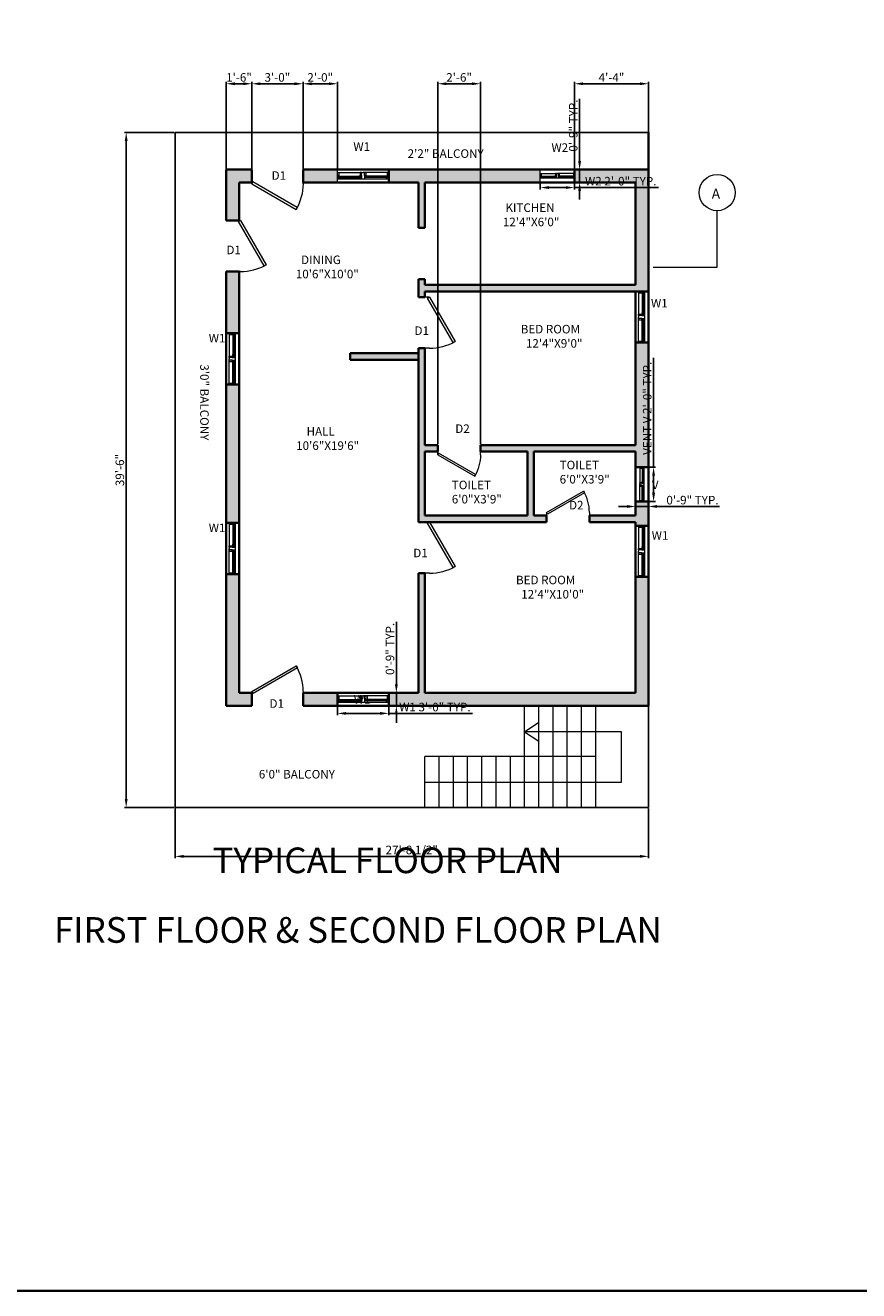
# Model space of a CAD drawing. Units: millimetres. Extents: x 50579 to 52843, y 62224 to 63803.
# Tile 3 of 5: x 51453 to 52038, y 62224 to 63113. Entities that reach past the tile are written whole.
import ezdxf

# ---------------------------------------------------------------- set-up
doc = ezdxf.new("R2010")
doc.units = ezdxf.units.MM
for name, color, linetype, lineweight in [('A-ANNO-DIMS', 2, 'Continuous', 18), ('A-ANNO-IDEN', 6, 'Continuous', 18), ('A-ANNO-SYMB', 6, 'Continuous', 18), ('A-ANNO-TITL', 4, 'Continuous', 25), ('A-ANNO-TTLB', 7, 'Continuous', 35), ('A-AREA-IDEN', 6, 'Continuous', 18), ('A-FLOR-BALC', 7, 'Continuous', 25), ('A-FLOR-STRS', 7, 'Continuous', 18), ('A-GLAZ', 4, 'Continuous', 18), ('A-WALL', 7, 'Continuous', 35), ('A-WALL-PATT', 251, 'Continuous', 13), ('DOOR', 20, 'Continuous', 18)]:
    doc.layers.add(name, color=color, linetype=linetype, lineweight=lineweight)
doc.styles.get("Standard").update_dxf_attribs({"font": 'arial.ttf'})
doc.dimstyles.new('ISO-25', dxfattribs={"dimtxt": 6, "dimasz": 6, "dimexe": 1.25, "dimexo": 0.625, "dimtad": 1, "dimdec": 0, "dimlunit": 3, "dimtxsty": 'Standard', "dimcen": 2.5, "dimadec": 0, "dimazin": 0, "dimtfac": 1, "dimtdec": 0, "dimtmove": 0, "dimatfit": 3, "dimfxl": 1, "dimarcsym": 0})

# ---------------------------------------------------------------- blocks, each defined once
blk = doc.blocks.new('W1')
for p, q in [((50927.56, 62719.85), (50945.56, 62719.85)), ((50927.56, 62717.25), (50944.56, 62717.25)), ((50927.56, 62716.35), (50944.56, 62716.35)), ((50927.56, 62715.35), (50963.56, 62715.35)), ((50929.58, 62717.08), (50942.53, 62717.08)), ((50929.58, 62716.8), (50942.53, 62716.8)), ((50929.58, 62716.54), (50942.53, 62716.54)), ((50944.56, 62717.61), (50944.56, 62715.35)), ((50963.56, 62719.85), (50945.56, 62719.85)), ((50946.56, 62717.61), (50946.56, 62715.35)), ((50963.56, 62717.25), (50946.56, 62717.25)), ((50963.56, 62716.35), (50946.56, 62716.35)), ((50961.53, 62717.08), (50948.58, 62717.08)), ((50961.53, 62716.8), (50948.58, 62716.8)), ((50961.53, 62716.54), (50948.58, 62716.54))]:
    blk.add_line(p, q)
for points in [[(50927.56, 62712.85), (50927.56, 62721.85), (50963.56, 62721.85), (50963.56, 62712.85)], [(50927.56, 62719.85), (50928.5, 62719.85), (50928.5, 62717.61), (50927.56, 62717.61)], [(50928.59, 62717.25), (50929.58, 62717.25), (50929.58, 62716.35), (50928.59, 62716.35)], [(50943.52, 62717.25), (50942.53, 62717.25), (50942.53, 62716.35), (50943.52, 62716.35)], [(50944.56, 62719.85), (50943.61, 62719.85), (50943.61, 62717.61), (50944.56, 62717.61)], [(50946.56, 62719.85), (50947.5, 62719.85), (50947.5, 62717.61), (50946.56, 62717.61)], [(50947.59, 62717.25), (50948.58, 62717.25), (50948.58, 62716.35), (50947.59, 62716.35)], [(50962.52, 62717.25), (50961.53, 62717.25), (50961.53, 62716.35), (50962.52, 62716.35)], [(50963.56, 62719.85), (50962.61, 62719.85), (50962.61, 62717.61), (50963.56, 62717.61)]]:
    blk.add_lwpolyline(points, close=True)
blk = doc.blocks.new('*U3')
for p, q in [((0, 0), (0, -6)), ((40, 0), (40, -6))]:
    blk.add_line(p, q)
blk.add_lwpolyline([(0, 0), (34.64, 20), (35.52, 18.48), (0.87, -1.52)], close=True)
blk.add_arc((0, 0), 40, 0, 30)
blk = doc.blocks.new('WIN-W2-PLAN')
for p, q in [((0, 6.16), (12, 6.16)), ((0, 4.43), (11.33, 4.43)), ((0, 3.83), (11.33, 3.83)), ((0, 3.16), (24, 3.16)), ((1.35, 4.32), (9.98, 4.32)), ((1.35, 4.13), (9.98, 4.13)), ((1.35, 3.95), (9.98, 3.95)), ((11.33, 4.67), (11.33, 3.16)), ((24, 6.16), (12, 6.16)), ((12.67, 4.67), (12.67, 3.16)), ((24, 4.43), (12.67, 4.43)), ((24, 3.83), (12.67, 3.83)), ((22.65, 4.32), (14.02, 4.32)), ((22.65, 4.13), (14.02, 4.13)), ((22.65, 3.95), (14.02, 3.95))]:
    blk.add_line(p, q)
for points in [[(0, 0), (0, 9), (24, 9), (24, 0)], [(0, 6.16), (0.63, 6.16), (0.63, 4.67), (0, 4.67)], [(0.69, 4.43), (1.35, 4.43), (1.35, 3.83), (0.69, 3.83)], [(10.64, 4.43), (9.98, 4.43), (9.98, 3.83), (10.64, 3.83)], [(11.33, 6.16), (10.7, 6.16), (10.7, 4.67), (11.33, 4.67)], [(12.67, 6.16), (13.29, 6.16), (13.29, 4.67), (12.67, 4.67)], [(13.36, 4.43), (14.02, 4.43), (14.02, 3.83), (13.36, 3.83)], [(23.31, 4.43), (22.65, 4.43), (22.65, 3.83), (23.31, 3.83)], [(24, 6.16), (23.37, 6.16), (23.37, 4.67), (24, 4.67)]]:
    blk.add_lwpolyline(points, close=True)
blk = doc.blocks.new('VENT-V-PLAN')
for p, q in [((2.84, 24), (2.84, 12)), ((4.57, 24), (4.57, 12.67)), ((4.68, 22.65), (4.68, 14.02)), ((4.87, 22.65), (4.87, 14.02)), ((5.05, 22.65), (5.05, 14.02)), ((5.17, 24), (5.17, 12.67)), ((5.84, 24), (5.84, 0)), ((2.84, 0), (2.84, 12)), ((4.33, 12.67), (5.84, 12.67)), ((4.33, 11.33), (5.84, 11.33)), ((4.57, 0), (4.57, 11.33)), ((4.68, 1.35), (4.68, 9.98)), ((4.87, 1.35), (4.87, 9.98)), ((5.05, 1.35), (5.05, 9.98)), ((5.17, 0), (5.17, 11.33))]:
    blk.add_line(p, q)
for points in [[(9, 24), (0, 24), (0, 0), (9, 0)], [(2.84, 24), (2.84, 23.37), (4.33, 23.37), (4.33, 24)], [(4.57, 23.31), (4.57, 22.65), (5.17, 22.65), (5.17, 23.31)], [(2.84, 12.67), (2.84, 13.3), (4.33, 13.3), (4.33, 12.67)], [(2.84, 11.33), (2.84, 10.71), (4.33, 10.71), (4.33, 11.33)], [(4.57, 13.36), (4.57, 14.02), (5.17, 14.02), (5.17, 13.36)], [(4.57, 10.64), (4.57, 9.98), (5.17, 9.98), (5.17, 10.64)], [(2.84, 0), (2.84, 0.63), (4.33, 0.63), (4.33, 0)], [(4.57, 0.69), (4.57, 1.35), (5.17, 1.35), (5.17, 0.69)]]:
    blk.add_lwpolyline(points, close=True)
blk = doc.blocks.new('STAIR-RETURN-PLAN')
for p, q in [((70, 0), (70, 71.5)), ((80, 0), (80, 71.5)), ((90, 0), (90, 71.5)), ((100, 0), (100, 71.5)), ((110, 0), (110, 71.5)), ((120, 0), (120, 71.5)), ((70, 53.25), (80, 59.99)), ((138.14, 53.25), (70, 53.25)), ((70, 53.25), (80, 46.5)), ((138.14, 17.87), (138.14, 53.25)), ((0, 0), (0, 35.75)), ((120, 35.75), (0, 35.75)), ((10, 0), (10, 35.75)), ((20, 0), (20, 35.75)), ((30, 0), (30, 35.75)), ((40, 0), (40, 35.75)), ((50, 0), (50, 35.75)), ((60, 0), (60, 35.75)), ((0, 17.87), (138.14, 17.87))]:
    blk.add_line(p, q)
blk = doc.blocks.new('*D27')
at = {"layer": 'A-ANNO-DIMS', "color": 0, "lineweight": -2, "transparency": 16777216}
for p, q in [((51671.96, 62634.23), (51671.96, 62628.2)), ((51707.96, 62634.23), (51707.96, 62628.2)), ((51677.96, 62629.45), (51701.96, 62629.45)), ((51707.96, 62629.45), (51766.93, 62629.45))]:
    blk.add_line(p, q, dxfattribs=at)
at = {"layer": 'A-ANNO-DIMS', "color": 0, "transparency": 16777216}
for points in [[(51677.96, 62630.45), (51677.96, 62628.45), (51671.96, 62629.45)], [(51701.96, 62630.45), (51701.96, 62628.45), (51707.96, 62629.45)]]:
    blk.add_solid(points, dxfattribs=at)
at = {"layer": 'Defpoints', "color": 0, "transparency": 16777216}
for p in [(51671.96, 62634.85), (51707.96, 62634.85), (51707.96, 62629.45)]:
    blk.add_point(p, dxfattribs=at)
at = {"layer": 'A-ANNO-DIMS', "color": 0, "transparency": 16777216, "insert": (51740.44, 62633.14), "char_height": 6, "attachment_point": 5}
blk.add_mtext('W1 3\'-0" TYP.', dxfattribs=at)
blk = doc.blocks.new('*D28')
at = {"layer": 'A-ANNO-DIMS', "color": 0, "lineweight": -2, "transparency": 16777216}
for p, q in [((51713.36, 62649.85), (51713.36, 62693.67)), ((51708.58, 62643.85), (51714.61, 62643.85)), ((51713.36, 62634.85), (51713.36, 62643.85)), ((51708.58, 62634.85), (51714.61, 62634.85)), ((51713.36, 62628.85), (51713.36, 62622.85))]:
    blk.add_line(p, q, dxfattribs=at)
at = {"layer": 'A-ANNO-DIMS', "color": 0, "transparency": 16777216}
for points in [[(51712.36, 62649.85), (51714.36, 62649.85), (51713.36, 62643.85)], [(51712.36, 62628.85), (51714.36, 62628.85), (51713.36, 62634.85)]]:
    blk.add_solid(points, dxfattribs=at)
at = {"layer": 'Defpoints', "color": 0, "transparency": 16777216}
for p in [(51707.96, 62643.85), (51713.36, 62643.85), (51707.96, 62634.85)]:
    blk.add_point(p, dxfattribs=at)
at = {"layer": 'A-ANNO-DIMS', "color": 0, "transparency": 16777216, "insert": (51709.67, 62674.76), "char_height": 6, "attachment_point": 5, "rotation": 90}
blk.add_mtext('0\'-9" TYP.', dxfattribs=at)
blk = doc.blocks.new('*D29')
at = {"layer": 'A-ANNO-DIMS', "color": 0, "lineweight": -2, "transparency": 16777216}
for p, q in [((51814.46, 63001.73), (51814.46, 62997.5)), ((51820.46, 62998.75), (51832.46, 62998.75)), ((51838.46, 63001.73), (51838.46, 62997.5)), ((51838.46, 62998.75), (51897.43, 62998.75))]:
    blk.add_line(p, q, dxfattribs=at)
at = {"layer": 'A-ANNO-DIMS', "color": 0, "transparency": 16777216}
for points in [[(51820.46, 62999.75), (51820.46, 62997.75), (51814.46, 62998.75)], [(51832.46, 62999.75), (51832.46, 62997.75), (51838.46, 62998.75)]]:
    blk.add_solid(points, dxfattribs=at)
at = {"layer": 'Defpoints', "color": 0, "transparency": 16777216}
for p in [(51814.46, 63002.35), (51838.46, 63002.35), (51838.46, 62998.75)]:
    blk.add_point(p, dxfattribs=at)
at = {"layer": 'A-ANNO-DIMS', "color": 0, "transparency": 16777216, "insert": (51870.94, 63002.44), "char_height": 6, "attachment_point": 5}
blk.add_mtext('W2 2\'-0" TYP.', dxfattribs=at)
blk = doc.blocks.new('*D30')
at = {"layer": 'A-ANNO-DIMS', "color": 0, "lineweight": -2, "transparency": 16777216}
for p, q in [((51842.06, 63017.35), (51842.06, 63061.17)), ((51839.08, 63011.35), (51843.31, 63011.35)), ((51842.06, 63002.35), (51842.06, 63011.35)), ((51839.08, 63002.35), (51843.31, 63002.35)), ((51842.06, 62996.35), (51842.06, 62990.35))]:
    blk.add_line(p, q, dxfattribs=at)
at = {"layer": 'A-ANNO-DIMS', "color": 0, "transparency": 16777216}
for points in [[(51841.06, 63017.35), (51843.06, 63017.35), (51842.06, 63011.35)], [(51841.06, 62996.35), (51843.06, 62996.35), (51842.06, 63002.35)]]:
    blk.add_solid(points, dxfattribs=at)
at = {"layer": 'Defpoints', "color": 0, "transparency": 16777216}
for p in [(51838.46, 63011.35), (51842.06, 63011.35), (51838.46, 63002.35)]:
    blk.add_point(p, dxfattribs=at)
at = {"layer": 'A-ANNO-DIMS', "color": 0, "transparency": 16777216, "insert": (51838.37, 63042.26), "char_height": 6, "attachment_point": 5, "rotation": 90}
blk.add_mtext('0\'-9" TYP.', dxfattribs=at)
blk = doc.blocks.new('*D31')
at = {"layer": 'A-ANNO-DIMS', "color": 0, "lineweight": -2, "transparency": 16777216}
for p, q in [((51894.02, 62802.37), (51894.02, 62879.11)), ((51891.04, 62802.37), (51895.27, 62802.37)), ((51894.02, 62784.37), (51894.02, 62796.37)), ((51891.04, 62778.37), (51895.27, 62778.37))]:
    blk.add_line(p, q, dxfattribs=at)
at = {"layer": 'A-ANNO-DIMS', "color": 0, "transparency": 16777216}
for points in [[(51893.02, 62796.37), (51895.02, 62796.37), (51894.02, 62802.37)], [(51893.02, 62784.37), (51895.02, 62784.37), (51894.02, 62778.37)]]:
    blk.add_solid(points, dxfattribs=at)
at = {"layer": 'Defpoints', "color": 0, "transparency": 16777216}
for p in [(51890.42, 62802.37), (51894.02, 62802.37), (51890.42, 62778.37)]:
    blk.add_point(p, dxfattribs=at)
at = {"layer": 'A-ANNO-DIMS', "color": 0, "transparency": 16777216, "insert": (51890.33, 62843.74), "char_height": 6, "attachment_point": 5, "rotation": 90}
blk.add_mtext('VENT V 2\'-0" TYP.', dxfattribs=at)
blk = doc.blocks.new('*D32')
at = {"layer": 'A-ANNO-DIMS', "color": 0, "lineweight": -2, "transparency": 16777216}
for p, q in [((51881.42, 62777.75), (51881.42, 62773.52)), ((51890.42, 62777.75), (51890.42, 62773.52)), ((51875.42, 62774.77), (51869.42, 62774.77)), ((51881.42, 62774.77), (51890.42, 62774.77)), ((51896.42, 62774.77), (51940.24, 62774.77))]:
    blk.add_line(p, q, dxfattribs=at)
at = {"layer": 'A-ANNO-DIMS', "color": 0, "transparency": 16777216}
for points in [[(51875.42, 62775.77), (51875.42, 62773.77), (51881.42, 62774.77)], [(51896.42, 62775.77), (51896.42, 62773.77), (51890.42, 62774.77)]]:
    blk.add_solid(points, dxfattribs=at)
at = {"layer": 'Defpoints', "color": 0, "transparency": 16777216}
for p in [(51881.42, 62778.37), (51890.42, 62778.37), (51890.42, 62774.77)]:
    blk.add_point(p, dxfattribs=at)
at = {"layer": 'A-ANNO-DIMS', "color": 0, "transparency": 16777216, "insert": (51921.33, 62778.46), "char_height": 6, "attachment_point": 5}
blk.add_mtext('0\'-9" TYP.', dxfattribs=at)
blk = doc.blocks.new('*D41')
at = {"layer": 'A-ANNO-DIMS', "color": 0, "lineweight": -2, "transparency": 16777216}
for p, q in [((51557.92, 62562.73), (51557.92, 62527.8)), ((51890.42, 62562.73), (51890.42, 62527.8)), ((51563.92, 62529.05), (51884.42, 62529.05))]:
    blk.add_line(p, q, dxfattribs=at)
at = {"layer": 'A-ANNO-DIMS', "color": 0, "transparency": 16777216}
for points in [[(51563.92, 62530.05), (51563.92, 62528.05), (51557.92, 62529.05)], [(51884.42, 62530.05), (51884.42, 62528.05), (51890.42, 62529.05)]]:
    blk.add_solid(points, dxfattribs=at)
at = {"layer": 'Defpoints', "color": 0, "transparency": 16777216}
for p in [(51557.92, 62563.35), (51890.42, 62563.35), (51890.42, 62529.05)]:
    blk.add_point(p, dxfattribs=at)
at = {"layer": 'A-ANNO-DIMS', "color": 0, "transparency": 16777216, "insert": (51724.17, 62532.78), "char_height": 6, "attachment_point": 5}
blk.add_mtext('27\'-8 1/2"', dxfattribs=at)
blk = doc.blocks.new('*D42')
at = {"layer": 'A-ANNO-DIMS', "color": 0, "lineweight": -2, "transparency": 16777216}
for p, q in [((51557.29, 63037.35), (51522.37, 63037.35)), ((51523.62, 62569.35), (51523.62, 63031.35)), ((51557.29, 62563.35), (51522.37, 62563.35))]:
    blk.add_line(p, q, dxfattribs=at)
at = {"layer": 'A-ANNO-DIMS', "color": 0, "transparency": 16777216}
for points in [[(51522.62, 63031.35), (51524.62, 63031.35), (51523.62, 63037.35)], [(51522.62, 62569.35), (51524.62, 62569.35), (51523.62, 62563.35)]]:
    blk.add_solid(points, dxfattribs=at)
at = {"layer": 'Defpoints', "color": 0, "transparency": 16777216}
for p in [(51523.62, 63037.35), (51557.92, 63037.35), (51557.92, 62563.35)]:
    blk.add_point(p, dxfattribs=at)
at = {"layer": 'A-ANNO-DIMS', "color": 0, "transparency": 16777216, "insert": (51519.93, 62800.35), "char_height": 6, "attachment_point": 5, "rotation": 90}
blk.add_mtext('39\'-6"', dxfattribs=at)
blk = doc.blocks.new('*D68')
at = {"layer": 'A-ANNO-DIMS', "color": 0, "lineweight": -2, "transparency": 16777216}
for p, q in [((51611.8, 63011.98), (51611.8, 63072.9)), ((51617.8, 63071.65), (51641.8, 63071.65)), ((51647.8, 63011.98), (51647.8, 63072.9))]:
    blk.add_line(p, q, dxfattribs=at)
at = {"layer": 'A-ANNO-DIMS', "color": 0, "transparency": 16777216}
for points in [[(51617.8, 63072.65), (51617.8, 63070.65), (51611.8, 63071.65)], [(51641.8, 63072.65), (51641.8, 63070.65), (51647.8, 63071.65)]]:
    blk.add_solid(points, dxfattribs=at)
at = {"layer": 'Defpoints', "color": 0, "transparency": 16777216}
for p in [(51647.8, 63071.65), (51611.8, 63011.35), (51647.8, 63011.35)]:
    blk.add_point(p, dxfattribs=at)
at = {"layer": 'A-ANNO-DIMS', "color": 0, "transparency": 16777216, "insert": (51629.8, 63075.34), "char_height": 6, "attachment_point": 5}
blk.add_mtext('3\'-0"', dxfattribs=at)
blk = doc.blocks.new('*D69')
at = {"layer": 'A-ANNO-DIMS', "color": 0, "lineweight": -2, "transparency": 16777216}
for p, q in [((51742.42, 62818.48), (51742.42, 63072.9)), ((51748.42, 63071.65), (51766.42, 63071.65)), ((51772.42, 62818.48), (51772.42, 63072.9))]:
    blk.add_line(p, q, dxfattribs=at)
at = {"layer": 'A-ANNO-DIMS', "color": 0, "transparency": 16777216}
for points in [[(51748.42, 63072.65), (51748.42, 63070.65), (51742.42, 63071.65)], [(51766.42, 63072.65), (51766.42, 63070.65), (51772.42, 63071.65)]]:
    blk.add_solid(points, dxfattribs=at)
at = {"layer": 'Defpoints', "color": 0, "transparency": 16777216}
for p in [(51772.42, 63071.65), (51742.42, 62817.85), (51772.42, 62817.85)]:
    blk.add_point(p, dxfattribs=at)
at = {"layer": 'A-ANNO-DIMS', "color": 0, "transparency": 16777216, "insert": (51757.42, 63075.34), "char_height": 6, "attachment_point": 5}
blk.add_mtext('2\'-6"', dxfattribs=at)
blk = doc.blocks.new('*D70')
at = {"layer": 'A-ANNO-DIMS', "color": 0, "lineweight": -2, "transparency": 16777216}
for p, q in [((51593.92, 63011.98), (51593.92, 63072.9)), ((51599.92, 63071.65), (51605.8, 63071.65)), ((51611.8, 63011.98), (51611.8, 63072.9))]:
    blk.add_line(p, q, dxfattribs=at)
at = {"layer": 'A-ANNO-DIMS', "color": 0, "transparency": 16777216}
for points in [[(51599.92, 63072.65), (51599.92, 63070.65), (51593.92, 63071.65)], [(51605.8, 63072.65), (51605.8, 63070.65), (51611.8, 63071.65)]]:
    blk.add_solid(points, dxfattribs=at)
at = {"layer": 'Defpoints', "color": 0, "transparency": 16777216}
for p in [(51611.8, 63071.65), (51593.92, 63011.35), (51611.8, 63011.35)]:
    blk.add_point(p, dxfattribs=at)
at = {"layer": 'A-ANNO-DIMS', "color": 0, "transparency": 16777216, "insert": (51602.86, 63075.34), "char_height": 6, "attachment_point": 5}
blk.add_mtext('1\'-6"', dxfattribs=at)
blk = doc.blocks.new('*D71')
at = {"layer": 'A-ANNO-DIMS', "color": 0, "lineweight": -2, "transparency": 16777216}
for p, q in [((51647.8, 63011.98), (51647.8, 63072.9)), ((51653.8, 63071.65), (51665.96, 63071.65)), ((51671.96, 63011.98), (51671.96, 63072.9))]:
    blk.add_line(p, q, dxfattribs=at)
at = {"layer": 'A-ANNO-DIMS', "color": 0, "transparency": 16777216}
for points in [[(51653.8, 63072.65), (51653.8, 63070.65), (51647.8, 63071.65)], [(51665.96, 63072.65), (51665.96, 63070.65), (51671.96, 63071.65)]]:
    blk.add_solid(points, dxfattribs=at)
at = {"layer": 'Defpoints', "color": 0, "transparency": 16777216}
for p in [(51671.96, 63071.65), (51647.8, 63011.35), (51671.96, 63011.35)]:
    blk.add_point(p, dxfattribs=at)
at = {"layer": 'A-ANNO-DIMS', "color": 0, "transparency": 16777216, "insert": (51659.88, 63075.34), "char_height": 6, "attachment_point": 5}
blk.add_mtext('2\'-0"', dxfattribs=at)
blk = doc.blocks.new('*D72')
at = {"layer": 'A-ANNO-DIMS', "color": 0, "lineweight": -2, "transparency": 16777216}
for p, q in [((51838.455361, 63011.976927), (51838.455361, 63072.901927)), ((51844.455361, 63071.651927), (51884.419171, 63071.651927)), ((51890.419171, 63011.976927), (51890.419171, 63072.901927))]:
    blk.add_line(p, q, dxfattribs=at)
at = {"layer": 'A-ANNO-DIMS', "color": 0, "transparency": 16777216}
for points in [[(51844.455361, 63072.651927), (51844.455361, 63070.651927), (51838.455361, 63071.651927)], [(51884.419171, 63072.651927), (51884.419171, 63070.651927), (51890.419171, 63071.651927)]]:
    blk.add_solid(points, dxfattribs=at)
at = {"layer": 'Defpoints', "color": 0, "transparency": 16777216}
for p in [(51890.419171, 63071.651927), (51838.455361, 63011.351927), (51890.419171, 63011.351927)]:
    blk.add_point(p, dxfattribs=at)
at = {"layer": 'A-ANNO-DIMS', "color": 0, "transparency": 16777216, "insert": (51864.437266, 63075.276927), "char_height": 6, "attachment_point": 5}
blk.add_mtext('4\'-4"', dxfattribs=at)

msp = doc.modelspace()

# ---------------------------------------------------------------- hatches: boundary and pattern name
at = {"layer": 'A-WALL-PATT'}
h = msp.add_hatch(color=256, dxfattribs=at)
h.dxf.hatch_style = 1
h.paths.add_polyline_path([(51611.8, 63006.85), (51611.8, 63011.35), (51593.92, 63011.35), (51593.92, 62975.7), (51602.92, 62975.7), (51602.92, 63002.35), (51611.8, 63002.35)])
h = msp.add_hatch(color=256, dxfattribs=at)
h.dxf.hatch_style = 1
h.paths.add_polyline_path([(51671.96, 63011.35), (51647.8, 63011.35), (51647.8, 63002.35), (51671.96, 63002.35)])
h = msp.add_hatch(color=256, dxfattribs=at)
h.dxf.hatch_style = 1
h.paths.add_polyline_path([(51814.46, 63011.35), (51707.96, 63011.35), (51707.96, 63002.35), (51728.92, 63002.35), (51728.92, 62970.35), (51733.42, 62970.35), (51733.42, 63002.35), (51814.46, 63002.35)])
h = msp.add_hatch(color=256, dxfattribs=at)
h.dxf.hatch_style = 1
h.paths.add_polyline_path([(51890.42, 63011.35), (51838.46, 63011.35), (51838.46, 63002.35), (51881.42, 63002.35), (51881.42, 62930.35), (51733.42, 62930.35), (51733.42, 62934.35), (51728.92, 62934.35), (51728.92, 62921.85), (51733.42, 62921.85), (51733.42, 62925.85), (51890.42, 62925.85)])
h = msp.add_hatch(color=256, dxfattribs=at)
h.dxf.hatch_style = 1
h.paths.add_polyline_path([(51602.92, 62939.7), (51598.42, 62939.7), (51593.92, 62939.7), (51593.92, 62896.5), (51602.92, 62896.5)])
h = msp.add_hatch(color=256, dxfattribs=at)
h.dxf.hatch_style = 1
h.paths.add_polyline_path([(51728.92, 62882.35), (51680.92, 62882.35), (51680.92, 62877.85), (51728.92, 62877.85)])
h = msp.add_hatch(color=256, dxfattribs=at)
h.dxf.hatch_style = 1
h.paths.add_polyline_path([(51733.42, 62885.85), (51731.17, 62885.85), (51728.92, 62885.85), (51728.92, 62763.85), (51818.92, 62763.85), (51818.92, 62768.35), (51809.92, 62768.35), (51809.92, 62813.35), (51881.42, 62813.35), (51881.42, 62802.37), (51890.42, 62802.37), (51890.42, 62889.85), (51881.42, 62889.85), (51881.42, 62817.85), (51772.42, 62817.85), (51772.42, 62813.35), (51805.42, 62813.35), (51805.42, 62768.35), (51733.42, 62768.35), (51733.42, 62813.35), (51742.42, 62813.35), (51742.42, 62815.6), (51742.42, 62817.85), (51733.42, 62817.85)])
h = msp.add_hatch(color=256, dxfattribs=at)
h.dxf.hatch_style = 1
h.paths.add_polyline_path([(51602.92, 62860.5), (51593.92, 62860.5), (51593.92, 62763.3), (51602.92, 62763.3)])
h = msp.add_hatch(color=256, dxfattribs=at)
h.dxf.hatch_style = 1
h.paths.add_polyline_path([(51890.42, 62778.37), (51881.42, 62778.37), (51881.42, 62768.35), (51848.92, 62768.35), (51848.92, 62763.85), (51881.42, 62763.85), (51881.42, 62761.3), (51890.42, 62761.3)])
h = msp.add_hatch(color=256, dxfattribs=at)
h.dxf.hatch_style = 1
h.paths.add_polyline_path([(51611.92, 62643.85), (51602.92, 62643.85), (51602.92, 62727.3), (51593.92, 62727.3), (51593.92, 62643.85), (51593.92, 62634.85), (51611.92, 62634.85)])
h = msp.add_hatch(color=256, dxfattribs=at)
h.dxf.hatch_style = 1
h.paths.add_polyline_path([(51890.42, 62725.3), (51881.42, 62725.3), (51881.42, 62643.85), (51733.42, 62643.85), (51733.42, 62727.85), (51728.92, 62727.85), (51728.92, 62643.85), (51707.96, 62643.85), (51707.96, 62634.85), (51890.42, 62634.85)])
h = msp.add_hatch(color=256, dxfattribs=at)
h.dxf.hatch_style = 1
h.paths.add_polyline_path([(51671.96, 62643.85), (51647.92, 62643.85), (51647.92, 62634.85), (51671.96, 62634.85)])

# ---------------------------------------------------------------- linework, layer by layer
at = {"layer": 'A-ANNO-SYMB'}
for p, q in [((51938.69, 62942.81), (51938.69, 62982.48)), ((51893.74, 62942.81), (51938.69, 62942.81))]:
    msp.add_line(p, q, dxfattribs=at)
msp.add_circle((51938.69, 62995.17), 12.7, dxfattribs=at)
at = {"layer": 'A-ANNO-TTLB'}
msp.add_lwpolyline([(50579.46, 63802.65), (52843.1, 63802.65), (52843.1, 62224.04), (50579.46, 62224.04)], close=True, dxfattribs=at)
at = {"layer": 'A-FLOR-BALC'}
for p, q in [((51557.92, 63037.35), (51890.42, 63037.35)), ((51557.92, 62563.35), (51557.92, 63037.35)), ((51890.42, 62634.85), (51890.42, 62563.35)), ((51890.42, 62563.35), (51557.92, 62563.35))]:
    msp.add_line(p, q, dxfattribs=at)
at = {"layer": 'A-WALL'}
for p, q in [((51890.42, 62634.85), (51890.42, 63037.35)), ((51593.92, 63011.35), (51611.8, 63011.35)), ((51593.92, 62975.7), (51593.92, 63011.35)), ((51611.8, 63002.35), (51611.8, 63011.35)), ((51647.8, 63011.35), (51890.42, 63011.35)), ((51647.8, 63002.35), (51647.8, 63011.35)), ((51707.96, 63011.35), (51707.96, 63002.35)), ((51838.46, 63011.35), (51838.46, 63002.35)), ((51602.92, 63002.35), (51611.8, 63002.35)), ((51602.92, 62975.7), (51602.92, 63002.35)), ((51647.8, 63002.35), (51728.92, 63002.35)), ((51728.92, 62970.35), (51728.92, 63002.35)), ((51733.42, 63002.35), (51881.42, 63002.35)), ((51733.42, 62970.35), (51733.42, 63002.35)), ((51881.42, 62930.35), (51881.42, 63002.35)), ((51593.92, 62975.7), (51602.92, 62975.7)), ((51728.92, 62970.35), (51733.42, 62970.35)), ((51593.92, 62643.85), (51593.92, 62939.7)), ((51593.92, 62939.7), (51602.92, 62939.7)), ((51602.92, 62877.85), (51602.92, 62939.7)), ((51728.92, 62934.35), (51733.42, 62934.35)), ((51728.92, 62921.85), (51728.92, 62934.35)), ((51733.42, 62930.35), (51733.42, 62934.35)), ((51733.42, 62930.35), (51881.42, 62930.35)), ((51733.42, 62925.85), (51890.42, 62925.85)), ((51733.42, 62921.85), (51733.42, 62925.85)), ((51881.42, 62817.85), (51881.42, 62925.85)), ((51728.92, 62921.85), (51733.42, 62921.85)), ((51593.92, 62896.5), (51602.92, 62896.5)), ((51680.92, 62882.35), (51728.92, 62882.35)), ((51680.92, 62877.85), (51680.92, 62882.35)), ((51728.92, 62885.85), (51733.42, 62885.85)), ((51728.92, 62763.85), (51728.92, 62885.85)), ((51733.42, 62817.85), (51733.42, 62885.85)), ((51881.42, 62889.85), (51890.42, 62889.85)), ((51602.92, 62643.85), (51602.92, 62877.85)), ((51680.92, 62877.85), (51728.92, 62877.85)), ((51593.92, 62860.5), (51602.92, 62860.5)), ((51733.42, 62817.85), (51742.42, 62817.85)), ((51733.42, 62813.35), (51742.42, 62813.35)), ((51733.42, 62768.35), (51733.42, 62813.35)), ((51742.42, 62813.35), (51742.42, 62817.85)), ((51772.42, 62817.85), (51881.42, 62817.85)), ((51772.42, 62813.35), (51772.42, 62817.85)), ((51772.42, 62813.35), (51805.42, 62813.35)), ((51805.42, 62768.35), (51805.42, 62813.35)), ((51809.92, 62813.35), (51881.42, 62813.35)), ((51809.92, 62768.35), (51809.92, 62813.35)), ((51881.42, 62768.35), (51881.42, 62813.35)), ((51881.42, 62802.37), (51890.42, 62802.37)), ((51881.42, 62778.37), (51890.42, 62778.37)), ((51733.42, 62768.35), (51805.42, 62768.35)), ((51809.92, 62768.35), (51818.92, 62768.35)), ((51818.92, 62768.35), (51818.92, 62763.85)), ((51848.92, 62768.35), (51881.42, 62768.35)), ((51848.92, 62768.35), (51848.92, 62763.85)), ((51593.92, 62763.3), (51602.92, 62763.3)), ((51728.92, 62763.85), (51818.92, 62763.85)), ((51848.92, 62763.85), (51881.42, 62763.85)), ((51881.42, 62643.85), (51881.42, 62763.85)), ((51881.42, 62761.3), (51890.42, 62761.3)), ((51593.92, 62727.3), (51602.92, 62727.3)), ((51728.92, 62727.85), (51733.42, 62727.85)), ((51728.92, 62643.85), (51728.92, 62727.85)), ((51733.42, 62643.85), (51733.42, 62727.85)), ((51881.42, 62725.3), (51890.42, 62725.3)), ((51593.92, 62634.85), (51593.92, 62643.85)), ((51602.92, 62643.85), (51611.92, 62643.85)), ((51611.92, 62643.85), (51611.92, 62634.85)), ((51647.92, 62643.85), (51647.92, 62634.85)), ((51647.92, 62643.85), (51728.92, 62643.85)), ((51671.96, 62643.85), (51671.96, 62634.85)), ((51707.96, 62643.85), (51707.96, 62634.85)), ((51733.42, 62643.85), (51881.42, 62643.85)), ((51593.92, 62634.85), (51611.92, 62634.85)), ((51647.92, 62634.85), (51890.42, 62634.85))]:
    msp.add_line(p, q, dxfattribs=at)

# ---------------------------------------------------------------- block references
at = {"layer": 'A-FLOR-STRS'}
msp.add_blockref('STAIR-RETURN-PLAN', (51733.42, 62563.35), dxfattribs=at)
at = {"layer": 'A-GLAZ'}
for name, p in [('W1', (744.4, 289.5)), ('WIN-W2-PLAN', (51814.46, 63002.35)), ('VENT-V-PLAN', (51881.42, 62778.37)), ('W1', (744.4, -78))]:
    msp.add_blockref(name, p, dxfattribs=at)
at = {"layer": 'A-GLAZ', "rotation": 90}
for p in [(114603.27, 11962.3), (114315.77, 11932.94), (114315.77, 11799.74), (114603.27, 11797.74)]:
    msp.add_blockref('W1', p, dxfattribs=at)
at = {"layer": 'DOOR'}
for p, xscale, yscale, zscale, rotation in [((51611.8, 63001.45), -0.9, 0.9, 0.9, 180), ((51603.82, 62975.7), 0.9, 0.9, 0.9, 270), ((51736.57, 62921.85), 0.9, 0.9, 0.9, 270), ((51742.42, 62811.1), -0.75, 0.75, 0.75, 180), ((51736.57, 62763.85), 0.9, 0.9, 0.9, 270)]:
    msp.add_blockref('*U3', p, dxfattribs=dict(at, xscale=xscale, yscale=yscale, zscale=zscale, rotation=rotation))
for p, xscale, yscale, zscale in [((51818.92, 62770.6), 0.7499999999998483, 0.7499999999998483, 0.7499999999998483), ((51611.92, 62644.75), 0.9, 0.9, 0.9)]:
    msp.add_blockref('*U3', p, dxfattribs=dict(at, xscale=xscale, yscale=yscale, zscale=zscale))

# ---------------------------------------------------------------- texts
at = {"layer": 'A-ANNO-IDEN', "char_height": 6, "attachment_point": 1}
for s, insert in [('  W1', (51683.17, 63030.53)), ('  W2', (51822.27, 63029.83)), ('  D1', (51622.07, 63010.21)), ('  D1', (51590.34, 62957.95)), ('  W1', (51892.2, 62920.52)), ('  D1', (51722.43, 62901.25)), ('  W1', (51581.59, 62895.97)), ('  D2', (51751.07, 62832.42)), ('  V', (51889.13, 62792.98)), ('  D2', (51830.98, 62778.71)), ('  W1', (51581.59, 62762.77)), ('  W1', (51892.7, 62757.41)), ('  D1', (51721.56, 62745.08)), ('  W1', (51683.43, 62642.29)), ('  D1', (51620.59, 62639.39))]:
    msp.add_mtext_dynamic_manual_height_columns(s, width=13.8936, gutter_width=12.5, heights=[0], dxfattribs=dict(at, insert=insert))
at = {"layer": 'A-ANNO-SYMB', "insert": (51930.61, 62998.01), "char_height": 7, "attachment_point": 1}
msp.add_mtext_dynamic_manual_height_columns('  A', width=13.8936, gutter_width=12.5, heights=[0], dxfattribs=at)
at = {"layer": 'A-ANNO-TITL', "char_height": 18, "attachment_point": 1}
for s, width, insert in [('  TYPICAL FLOOR PLAN', 341.9217, (51573.18, 62535.27)), ('  FIRST FLOOR & SECOND FLOOR PLAN', 623.0346, (51461.91, 62486.37))]:
    msp.add_mtext_dynamic_manual_height_columns(s, width=width, gutter_width=12.5, heights=[0], dxfattribs=dict(at, insert=insert))
at = {"layer": 'A-AREA-IDEN', "char_height": 6, "attachment_point": 1}
for s, width, insert in [('  2\'2" BALCONY', 88.9546, (51717.6, 63025.62)), ('  KITCHEN\\P 12\'4"X6\'0"', 46.1696, (51786.31, 62987.6)), ('  DINING\\P10\'6"X10\'0"', 46.1696, (51642.75, 62951.01)), ('  BED ROOM \\P    12\'4"X9\'0"', 60.368, (51797.03, 62902.32)), ('    HALL\\P10\'6"X19\'6"', 46.1696, (51642.98, 62830.5)), ('  TOILET\\P  6\'0"X3\'9"', 46.1696, (51824.38, 62806.89)), ('  TOILET\\P  6\'0"X3\'9"', 46.1696, (51748.63, 62792.9)), ('  BED ROOM \\P    12\'4"X10\'0"', 60.368, (51793.71, 62726.14)), ('  6\'0" BALCONY', 88.9546, (51613.1, 62589.74))]:
    msp.add_mtext_dynamic_manual_height_columns(s, width=width, gutter_width=12.5, heights=[0], dxfattribs=dict(at, insert=insert))
at = {"layer": 'A-AREA-IDEN', "insert": (51581.59, 62878.29), "char_height": 6, "attachment_point": 1, "rotation": 270}
msp.add_mtext_dynamic_manual_height_columns('  3\'0" BALCONY', width=88.9546, gutter_width=12.5, heights=[0], dxfattribs=at)

# ---------------------------------------------------------------- dimensions: what is measured, and where the dimension line sits
at = {"layer": 'A-ANNO-DIMS'}
for base, p1, p2, picture, middle in [((51611.8, 63071.65), (51593.92, 63011.35), (51611.8, 63011.35), '*D70', (51602.86, 63075.34)), ((51647.8, 63071.65), (51611.8, 63011.35), (51647.8, 63011.35), '*D68', (51629.8, 63075.34)), ((51671.96, 63071.65), (51647.8, 63011.35), (51671.96, 63011.35), '*D71', (51659.88, 63075.34)), ((51772.42, 63071.65), (51742.42, 62817.85), (51772.42, 62817.85), '*D69', (51757.42, 63075.34)), ((51890.42, 63071.65), (51838.46, 63011.35), (51890.42, 63011.35), '*D72', (51864.44, 63075.28)), ((51890.42, 62529.05), (51557.92, 62563.35), (51890.42, 62563.35), '*D41', (51724.17, 62532.78))]:
    dim = msp.add_linear_dim(base=base, p1=p1, p2=p2, dimstyle='ISO-25', override={"dimdec": 1, "dimlfac": 1, "dimrnd": 0, "dimzin": 1, "dimdsep": 46, "dimlunit": 4, "dimfrac": 2}, dxfattribs=at)
    dim.commit()
    dim.dimension.update_dxf_attribs({"geometry": picture, "text_midpoint": middle})
for base, p1, p2, text, picture, middle in [((51842.06, 63011.35), (51838.46, 63002.35), (51838.46, 63011.35), '<> TYP.', '*D30', (51838.37, 63042.26)), ((51894.02, 62802.37), (51890.42, 62778.37), (51890.42, 62802.37), 'VENT V <> TYP.', '*D31', (51890.33, 62843.74)), ((51713.36, 62643.85), (51707.96, 62634.85), (51707.96, 62643.85), '<> TYP.', '*D28', (51709.67, 62674.76))]:
    dim = msp.add_linear_dim(base=base, p1=p1, p2=p2, angle=90, text=text, dimstyle='ISO-25', override={"dimdec": 1, "dimlfac": 1, "dimrnd": 0, "dimzin": 1, "dimdsep": 46, "dimlunit": 4, "dimfrac": 2}, dxfattribs=at)
    dim.commit()
    dim.dimension.update_dxf_attribs({"geometry": picture, "text_midpoint": middle})
dim = msp.add_linear_dim(base=(51523.62, 63037.35), p1=(51557.92, 62563.35), p2=(51557.92, 63037.35), angle=90, dimstyle='ISO-25', override={"dimdec": 1, "dimlfac": 1, "dimrnd": 0, "dimzin": 1, "dimdsep": 46, "dimlunit": 4, "dimfrac": 2}, dxfattribs=at)
dim.commit()
dim.dimension.update_dxf_attribs({"geometry": '*D42', "text_midpoint": (51519.93, 62800.35)})
for base, p1, p2, text, picture, middle in [((51838.46, 62998.75), (51814.46, 63002.35), (51838.46, 63002.35), 'W2 <> TYP.', '*D29', (51870.94, 63002.44)), ((51890.42, 62774.77), (51881.42, 62778.37), (51890.42, 62778.37), '<> TYP.', '*D32', (51921.33, 62778.46)), ((51707.96, 62629.45), (51671.96, 62634.85), (51707.96, 62634.85), 'W1 <> TYP.', '*D27', (51740.44, 62633.14))]:
    dim = msp.add_linear_dim(base=base, p1=p1, p2=p2, text=text, dimstyle='ISO-25', override={"dimdec": 1, "dimlfac": 1, "dimrnd": 0, "dimzin": 1, "dimdsep": 46, "dimlunit": 4, "dimfrac": 2}, dxfattribs=at)
    dim.commit()
    dim.dimension.update_dxf_attribs({"geometry": picture, "text_midpoint": middle})

doc.saveas('drawing.dxf')
